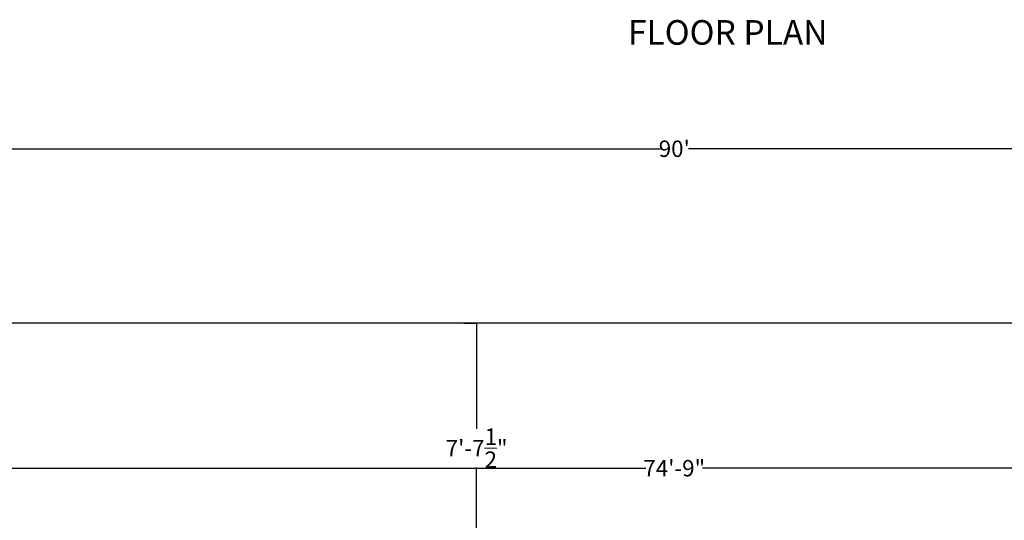
# Model space of a CAD drawing. Units: inches. Extents: x -2181 to 1225, y -80 to 4016.
# Tile 5 of 10: x 308 to 668, y 592 to 775. Entities that reach past the tile are written whole.
import ezdxf

# ---------------------------------------------------------------- set-up
doc = ezdxf.new("R2010")
doc.units = ezdxf.units.IN
doc.header["$MEASUREMENT"] = 0
for name, color, linetype, lineweight in [('A-ANNO-DIMS', 2, 'Continuous', 18), ('A-ANNO-TEXT', 7, 'Continuous', 18), ('C-PROP', 7, 'Continuous', 30)]:
    doc.layers.add(name, color=color, linetype=linetype, lineweight=lineweight)
doc.styles.get("Standard").update_dxf_attribs({"font": 'arial.ttf'})
doc.dimstyles.get("Standard").update_dxf_attribs({"dimtxt": 6, "dimasz": 0.18, "dimexe": 0.18, "dimexo": 0.0625, "dimgap": 0.09, "dimtad": 0, "dimtih": 1, "dimtoh": 1, "dimdec": 4, "dimzin": 0, "dimdsep": 46, "dimlunit": 4, "dimtxsty": 'Standard', "dimcen": 0.09, "dimadec": 0, "dimazin": 0, "dimtfac": 1, "dimtdec": 4, "dimtofl": 0, "dimtmove": 0, "dimatfit": 3, "dimfxl": 1, "dimtolj": 1, "dimtzin": 0, "dimarcsym": 0})

# ---------------------------------------------------------------- blocks, each defined once
blk = doc.blocks.new('*D22')
at = {"layer": 'A-ANNO-DIMS', "color": 0, "lineweight": -2, "transparency": 16777216}
for p, q in [((470.02, 664.48), (474.9, 664.48)), ((474.72, 664.3), (474.72, 625.85)), ((474.72, 573.16), (474.72, 611.62)), ((624.01, 572.98), (474.54, 572.98))]:
    blk.add_line(p, q, dxfattribs=at)
at = {"layer": 'A-ANNO-DIMS', "color": 0, "transparency": 16777216}
for points in [[(474.69, 664.3), (474.75, 664.3), (474.72, 664.48)], [(474.69, 573.16), (474.75, 573.16), (474.72, 572.98)]]:
    blk.add_solid(points, dxfattribs=at)
at = {"layer": 'Defpoints', "color": 0, "transparency": 16777216}
for p in [(469.95, 664.48), (474.72, 572.98), (624.08, 572.98)]:
    blk.add_point(p, dxfattribs=at)
at = {"layer": 'A-ANNO-DIMS', "color": 0, "transparency": 16777216, "insert": (474.72, 618.73), "char_height": 6, "attachment_point": 5}
blk.add_mtext('\\A1;7\'-7{\\H1x;\\S1/2;}"', dxfattribs=at)
blk = doc.blocks.new('*D70')
at = {"layer": 'A-ANNO-DIMS', "color": 0, "lineweight": -2, "transparency": 16777216}
for p, q in [((7.01, 664.55), (7.01, 728.44)), ((7.19, 728.26), (541.83, 728.26)), ((1086.83, 728.26), (552.2, 728.26)), ((1087.01, 664.55), (1087.01, 728.44))]:
    blk.add_line(p, q, dxfattribs=at)
at = {"layer": 'A-ANNO-DIMS', "color": 0, "transparency": 16777216}
for points in [[(7.19, 728.29), (7.19, 728.23), (7.01, 728.26)], [(1086.83, 728.29), (1086.83, 728.23), (1087.01, 728.26)]]:
    blk.add_solid(points, dxfattribs=at)
at = {"layer": 'Defpoints', "color": 0, "transparency": 16777216}
for p in [(1087.01, 728.26), (7.01, 664.48), (1087.01, 664.48)]:
    blk.add_point(p, dxfattribs=at)
at = {"layer": 'A-ANNO-DIMS', "color": 0, "transparency": 16777216, "insert": (547.01, 728.26), "char_height": 6, "attachment_point": 5}
blk.add_mtext("\\A1;90'", dxfattribs=at)
blk = doc.blocks.new('*D71')
at = {"layer": 'A-ANNO-DIMS', "color": 0, "lineweight": -2, "transparency": 16777216}
for p, q in [((98.51, 573.05), (98.51, 611.58)), ((98.69, 611.4), (536.64, 611.4)), ((995.33, 611.4), (557.39, 611.4)), ((995.51, 573.05), (995.51, 611.58))]:
    blk.add_line(p, q, dxfattribs=at)
at = {"layer": 'A-ANNO-DIMS', "color": 0, "transparency": 16777216}
for points in [[(98.69, 611.43), (98.69, 611.37), (98.51, 611.4)], [(995.33, 611.43), (995.33, 611.37), (995.51, 611.4)]]:
    blk.add_solid(points, dxfattribs=at)
at = {"layer": 'Defpoints', "color": 0, "transparency": 16777216}
for p in [(995.51, 611.4), (98.51, 572.98), (995.51, 572.98)]:
    blk.add_point(p, dxfattribs=at)
at = {"layer": 'A-ANNO-DIMS', "color": 0, "transparency": 16777216, "insert": (547.01, 611.4), "char_height": 6, "attachment_point": 5}
blk.add_mtext('\\A1;74\'-9"', dxfattribs=at)

msp = doc.modelspace()

# ---------------------------------------------------------------- linework, layer by layer
at = {"layer": 'C-PROP'}
msp.add_lwpolyline([(1087.01461, 16.48479), (1087.01461, 664.48479), (7.01461, 664.48479), (7.01461, 16.48479)], dxfattribs=at)

# ---------------------------------------------------------------- texts
at = {"layer": 'A-ANNO-TEXT', "insert": (530.07831, 775.30041), "char_height": 9, "attachment_point": 1}
msp.add_mtext_dynamic_manual_height_columns('FLOOR PLAN ', width=291.4178321, gutter_width=1, heights=[0], dxfattribs=at)

# ---------------------------------------------------------------- dimensions: what is measured, and where the dimension line sits
at = {"layer": 'A-ANNO-DIMS'}
for base, p1, p2, picture, middle in [((1087.01461, 728.26231), (7.01461, 664.48479), (1087.01461, 664.48479), '*D70', (547.01461, 728.26231)), ((995.51461, 611.40365), (98.51461, 572.98479), (995.51461, 572.98479), '*D71', (547.01461, 611.40365))]:
    dim = msp.add_linear_dim(base=base, p1=p1, p2=p2, dimstyle='Standard', override={"dimclrd": 0, "dimclre": 0, "dimclrt": 0}, dxfattribs=at)
    dim.commit()
    dim.dimension.update_dxf_attribs({"geometry": picture, "text_midpoint": middle})
dim = msp.add_linear_dim(base=(474.72038, 572.98479), p1=(469.95283, 664.48479), p2=(624.07639, 572.98479), angle=90, dimstyle='Standard', override={"dimclrd": 0, "dimclre": 0, "dimclrt": 0}, dxfattribs=at)
dim.commit()
dim.dimension.update_dxf_attribs({"geometry": '*D22', "text_midpoint": (474.72038, 618.73479)})

doc.saveas('drawing.dxf')
